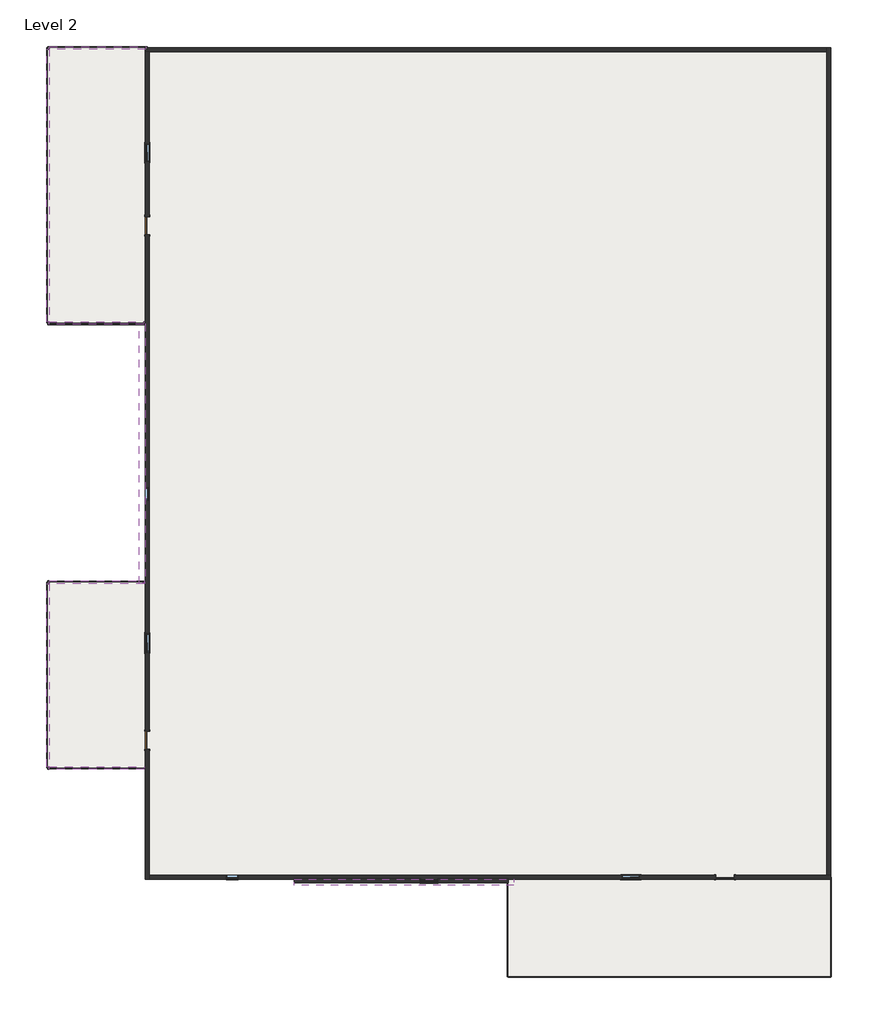
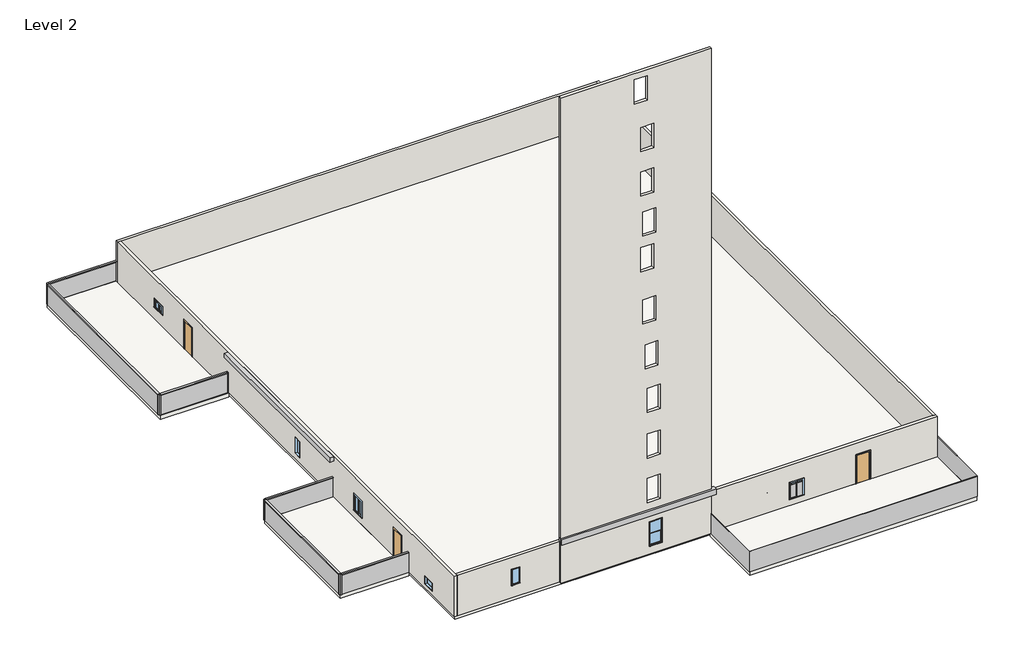
# One storey: 16 members, 10 plates, 7 windows, 5 walls, 4 slabs, 3 doors, 2 proxies.
"""IFC4 building model written with IfcOpenShell, lengths in millimetres."""

from ifc_helpers import new_model, si_unit, frame, origin, place, context, project, spatial, polyline, outline, extrude, faceted_brep, transform, mapped, element, save
from components import generic_models_11_generic_models_11_cbfe9a59, generic_models_22_generic_models_22_0e0807fa, door_54dd4da4, door_719f80de, member_4491d118, member_5d32774f, member_6474a55f, member_23f0e500, member_8787ee90, member_8a2e7db5, system_panel_glazed_dbf8c7ac, system_panel_glazed_64af9de3, system_panel_glazed_abcfc967, system_panel_glazed_a32a2426, system_panel_glazed_9b7d9a9b, system_panel_glazed_6b509a71, system_panel_glazed_fce9463a, system_panel_glazed_0e25fa2a, window_f274a882, window_80bd9af0, window_57c3ee1c, window_78885257, window_a4355bb3, window_54100e87

model = new_model("IFC4")

# Units and contexts
model_context = context("Model", 3, world=origin())
ifc_project = project(units=[si_unit("LENGTHUNIT", "METRE", prefix="MILLI")], contexts=[model_context])

# Site, building, storey
site = spatial("IfcSite", under=ifc_project)
building = spatial("IfcBuilding", under=site)
storey = spatial("IfcBuildingStorey", under=building, Name="Level 2", Elevation=3048.0)

# Proxies
placement = place(None, origin())
generic_models_11_generic_models_11_shape = generic_models_11_generic_models_11_cbfe9a59(model_context)
element("IfcBuildingElementProxy", 1, Name="Generic Models 11 : Generic Models 11", ObjectType="Generic Models 11 : Generic Models 11", at=placement, inside=storey, context=model_context, shape_type="MappedRepresentation", body=[
    mapped(generic_models_11_generic_models_11_shape, transform((0.0, 0.0, 0.0), x_axis=(1.0, 0.0, 0.0), y_axis=(0.0, 1.0, 0.0), z_axis=(0.0, 0.0, 1.0))),
])
generic_models_22_generic_models_22_shape = generic_models_22_generic_models_22_0e0807fa(model_context)
element("IfcBuildingElementProxy", 2, Name="Generic Models 22 : Generic Models 22", ObjectType="Generic Models 22 : Generic Models 22", at=placement, inside=storey, context=model_context, shape_type="MappedRepresentation", body=[
    mapped(generic_models_22_generic_models_22_shape, transform((0.0, 0.0, 0.0), x_axis=(1.0, 0.0, 0.0), y_axis=(0.0, 1.0, 0.0), z_axis=(0.0, 0.0, 1.0))),
])

# Doors
door_shape = door_54dd4da4(model_context)
element("IfcDoor", 3, ObjectType="Single-Flush : 36\" x 84\"", at=placement, inside=storey, context=model_context, shape_type="MappedRepresentation", body=[
    mapped(door_shape, transform((-15073.438074, -13886.1985361, 3048.0), x_axis=(0.0, 1.0, 0.0), y_axis=(-1.0, 0.0, 0.0), z_axis=(0.0, 0.0, 1.0))),
])
door_2_shape = door_719f80de(model_context)
element("IfcDoor", 4, ObjectType="Single-Flush : 36\" x 84\"", at=placement, inside=storey, context=model_context, shape_type="MappedRepresentation", body=[
    mapped(door_2_shape, transform((-15073.438074, 11900.6871782, 3048.0), x_axis=(0.0, -1.0, 0.0), y_axis=(1.0, 0.0, 0.0), z_axis=(0.0, 0.0, 1.0))),
])
element("IfcDoor", 5, ObjectType="Single-Flush : 36\" x 84\"", at=placement, inside=storey, context=model_context, shape_type="MappedRepresentation", body=[
    mapped(door_2_shape, transform((13882.561926, -20744.1985361, 3048.0), x_axis=(1.0, 0.0, 0.0), y_axis=(0.0, 1.0, 0.0), z_axis=(0.0, 0.0, 1.0))),
])

# Members
member_shape = member_4491d118(model_context)
element("IfcMember", 6, ObjectType="Rectangular Mullion : 2.5\" x 5\" rectangular", at=placement, inside=storey, context=model_context, shape_type="MappedRepresentation", body=[
    mapped(member_shape, transform((-20051.838074, 20810.2014639, 3048.0), x_axis=(0.0, 1.0, 0.0), y_axis=(1.0, 0.0, 0.0), z_axis=(0.0, 0.0, -1.0))),
])
element("IfcMember", 7, ObjectType="Rectangular Mullion : 2.5\" x 5\" rectangular", at=placement, inside=storey, context=model_context, shape_type="MappedRepresentation", body=[
    mapped(member_shape, transform((-15073.438074, 20810.2014639, 3048.0), x_axis=(1.0, 0.0, 0.0), y_axis=(0.0, -1.0, 0.0), z_axis=(0.0, 0.0, -1.0))),
])
element("IfcMember", 8, ObjectType="Rectangular Mullion : 2.5\" x 5\" rectangular", at=placement, inside=storey, context=model_context, shape_type="MappedRepresentation", body=[
    mapped(member_shape, transform((-20051.838074, 7023.8871782, 3048.0), x_axis=(-1.0, 0.0, 0.0), y_axis=(0.0, 1.0, 0.0), z_axis=(0.0, 0.0, -1.0))),
])
element("IfcMember", 9, ObjectType="Rectangular Mullion : 2.5\" x 5\" rectangular", at=placement, inside=storey, context=model_context, shape_type="MappedRepresentation", body=[
    mapped(member_shape, transform((-20051.838074, -5966.8213044, 3048.0), x_axis=(0.0, 1.0, 0.0), y_axis=(1.0, 0.0, 0.0), z_axis=(0.0, 0.0, -1.0))),
])
element("IfcMember", 10, ObjectType="Rectangular Mullion : 2.5\" x 5\" rectangular", at=placement, inside=storey, context=model_context, shape_type="MappedRepresentation", body=[
    mapped(member_shape, transform((-20051.838074, -15263.2213044, 3048.0), x_axis=(-1.0, 0.0, 0.0), y_axis=(0.0, 1.0, 0.0), z_axis=(0.0, 0.0, -1.0))),
])
element("IfcMember", 11, ObjectType="Rectangular Mullion : 2.5\" x 5\" rectangular", at=placement, inside=storey, context=model_context, shape_type="MappedRepresentation", body=[
    mapped(member_shape, transform((-20051.838074, 20810.2014639, 4572.0), x_axis=(-1.0, 0.0, 0.0), y_axis=(0.0, -1.0, 0.0), z_axis=(0.0, 0.0, 1.0))),
])
element("IfcMember", 12, ObjectType="Rectangular Mullion : 2.5\" x 5\" rectangular", at=placement, inside=storey, context=model_context, shape_type="MappedRepresentation", body=[
    mapped(member_shape, transform((-20051.838074, 7023.8871782, 4572.0), x_axis=(0.0, -1.0, 0.0), y_axis=(1.0, 0.0, 0.0), z_axis=(0.0, 0.0, 1.0))),
])
element("IfcMember", 13, ObjectType="Rectangular Mullion : 2.5\" x 5\" rectangular", at=placement, inside=storey, context=model_context, shape_type="MappedRepresentation", body=[
    mapped(member_shape, transform((-20051.838074, -5966.8213044, 4572.0), x_axis=(-1.0, 0.0, 0.0), y_axis=(0.0, -1.0, 0.0), z_axis=(0.0, 0.0, 1.0))),
])
element("IfcMember", 14, ObjectType="Rectangular Mullion : 2.5\" x 5\" rectangular", at=placement, inside=storey, context=model_context, shape_type="MappedRepresentation", body=[
    mapped(member_shape, transform((-20051.838074, -15263.2213044, 4572.0), x_axis=(0.0, -1.0, 0.0), y_axis=(1.0, 0.0, 0.0), z_axis=(0.0, 0.0, 1.0))),
])
element("IfcMember", 15, ObjectType="Rectangular Mullion : 2.5\" x 5\" rectangular", at=placement, inside=storey, context=model_context, shape_type="MappedRepresentation", body=[
    mapped(member_shape, transform((-15175.038074, 7023.8871782, 4572.0), x_axis=(1.0, 0.0, 0.0), y_axis=(0.0, 1.0, 0.0), z_axis=(0.0, 0.0, 1.0))),
])
member_2_shape = member_5d32774f(model_context)
element("IfcMember", 16, ObjectType="Rectangular Mullion : 2.5\" x 5\" rectangular", at=placement, inside=storey, context=model_context, shape_type="MappedRepresentation", body=[
    mapped(member_2_shape, transform((-15136.938074, 20810.2014639, 4572.0), x_axis=(0.0, 0.0, 1.0), y_axis=(0.0, -1.0, 0.0), z_axis=(1.0, 0.0, 0.0))),
])
member_3_shape = member_6474a55f(model_context)
element("IfcMember", 17, ObjectType="Rectangular Mullion : 2.5\" x 5\" rectangular", at=placement, inside=storey, context=model_context, shape_type="MappedRepresentation", body=[
    mapped(member_3_shape, transform((-20051.838074, 20746.7014639, 4572.0), x_axis=(0.0, 0.0, 1.0), y_axis=(1.0, 0.0, 0.0), z_axis=(0.0, 1.0, 0.0))),
])
member_4_shape = member_23f0e500(model_context)
element("IfcMember", 18, ObjectType="Rectangular Mullion : 2.5\" x 5\" rectangular", at=placement, inside=storey, context=model_context, shape_type="MappedRepresentation", body=[
    mapped(member_4_shape, transform((-15230.4716465, -5966.8213044, 4572.0), x_axis=(0.0, 0.0, 1.0), y_axis=(0.0, -1.0, 0.0), z_axis=(1.0, 0.0, 0.0))),
])
member_5_shape = member_8787ee90(model_context)
element("IfcMember", 19, ObjectType="Rectangular Mullion : 2.5\" x 5\" rectangular", at=placement, inside=storey, context=model_context, shape_type="MappedRepresentation", body=[
    mapped(member_5_shape, transform((-20051.838074, -6030.3213044, 4572.0), x_axis=(0.0, 0.0, 1.0), y_axis=(1.0, 0.0, 0.0), z_axis=(0.0, 1.0, 0.0))),
])
element("IfcMember", 20, ObjectType="Rectangular Mullion : 2.5\" x 5\" rectangular", at=placement, inside=storey, context=model_context, shape_type="MappedRepresentation", body=[
    mapped(member_4_shape, transform((-19988.338074, -15263.2213044, 4572.0), x_axis=(0.0, 0.0, 1.0), y_axis=(0.0, 1.0, 0.0), z_axis=(-1.0, 0.0, 0.0))),
])
member_6_shape = member_8a2e7db5(model_context)
element("IfcMember", 21, ObjectType="Rectangular Mullion : 2.5\" x 5\" rectangular", at=placement, inside=storey, context=model_context, shape_type="MappedRepresentation", body=[
    mapped(member_6_shape, transform((-19988.338074, 7023.8871782, 4572.0), x_axis=(0.0, 0.0, 1.0), y_axis=(0.0, 1.0, 0.0), z_axis=(-1.0, 0.0, 0.0))),
])

# Plates
system_panel_glazed_shape = system_panel_glazed_dbf8c7ac(model_context)
element("IfcPlate", 22, ObjectType="System Panel : Glazed", at=placement, inside=storey, context=model_context, shape_type="MappedRepresentation", body=[
    mapped(system_panel_glazed_shape, transform((11088.561926, -20845.7985361, 3048.0), x_axis=(1.0, 0.0, 0.0), y_axis=(0.0, 1.0, 0.0), z_axis=(0.0, 0.0, 1.0))),
])
element("IfcPlate", 23, ObjectType="System Panel : Glazed", at=placement, inside=storey, context=model_context, shape_type="MappedRepresentation", body=[
    mapped(system_panel_glazed_shape, transform((11088.561926, -25722.5985361, 3048.0), x_axis=(-1.0, 0.0, 0.0), y_axis=(0.0, -1.0, 0.0), z_axis=(0.0, 0.0, 1.0))),
])
system_panel_glazed_2_shape = system_panel_glazed_64af9de3(model_context)
element("IfcPlate", 24, ObjectType="System Panel : Glazed", at=placement, inside=storey, context=model_context, shape_type="MappedRepresentation", body=[
    mapped(system_panel_glazed_2_shape, transform((19165.761926, -23233.3985361, 3048.0), x_axis=(0.0, -1.0, 0.0), y_axis=(1.0, 0.0, 0.0), z_axis=(0.0, 0.0, 1.0))),
])
system_panel_glazed_3_shape = system_panel_glazed_abcfc967(model_context)
element("IfcPlate", 25, ObjectType="System Panel : Glazed", at=placement, inside=storey, context=model_context, shape_type="MappedRepresentation", body=[
    mapped(system_panel_glazed_3_shape, transform((3011.361926, -23273.4060583, 3048.0), x_axis=(0.0, 1.0, 0.0), y_axis=(-1.0, 0.0, 0.0), z_axis=(0.0, 0.0, 1.0))),
])
system_panel_glazed_4_shape = system_panel_glazed_a32a2426(model_context)
element("IfcPlate", 26, ObjectType="System Panel : Glazed", at=placement, inside=storey, context=model_context, shape_type="MappedRepresentation", body=[
    mapped(system_panel_glazed_4_shape, transform((-17562.638074, 20810.2014639, 3048.0), x_axis=(1.0, 0.0, 0.0), y_axis=(0.0, 1.0, 0.0), z_axis=(0.0, 0.0, 1.0))),
])
system_panel_glazed_5_shape = system_panel_glazed_9b7d9a9b(model_context)
element("IfcPlate", 27, ObjectType="System Panel : Glazed", at=placement, inside=storey, context=model_context, shape_type="MappedRepresentation", body=[
    mapped(system_panel_glazed_5_shape, transform((-20051.838074, 13917.0443211, 3048.0), x_axis=(0.0, 1.0, 0.0), y_axis=(-1.0, 0.0, 0.0), z_axis=(0.0, 0.0, 1.0))),
])
system_panel_glazed_6_shape = system_panel_glazed_6b509a71(model_context)
element("IfcPlate", 28, ObjectType="System Panel : Glazed", at=placement, inside=storey, context=model_context, shape_type="MappedRepresentation", body=[
    mapped(system_panel_glazed_6_shape, transform((-17609.4048602, -5966.8213044, 3048.0), x_axis=(1.0, 0.0, 0.0), y_axis=(0.0, 1.0, 0.0), z_axis=(0.0, 0.0, 1.0))),
])
element("IfcPlate", 29, ObjectType="System Panel : Glazed", at=placement, inside=storey, context=model_context, shape_type="MappedRepresentation", body=[
    mapped(system_panel_glazed_6_shape, transform((-17609.4048602, -15263.2213044, 3048.0), x_axis=(-1.0, 0.0, 0.0), y_axis=(0.0, -1.0, 0.0), z_axis=(0.0, 0.0, 1.0))),
])
system_panel_glazed_7_shape = system_panel_glazed_fce9463a(model_context)
element("IfcPlate", 30, ObjectType="System Panel : Glazed", at=placement, inside=storey, context=model_context, shape_type="MappedRepresentation", body=[
    mapped(system_panel_glazed_7_shape, transform((-20051.838074, -10615.0213044, 3048.0), x_axis=(0.0, 1.0, 0.0), y_axis=(-1.0, 0.0, 0.0), z_axis=(0.0, 0.0, 1.0))),
])
system_panel_glazed_8_shape = system_panel_glazed_0e25fa2a(model_context)
element("IfcPlate", 31, ObjectType="System Panel : Glazed", at=placement, inside=storey, context=model_context, shape_type="MappedRepresentation", body=[
    mapped(system_panel_glazed_8_shape, transform((-17613.438074, 7023.8871782, 3048.0), x_axis=(-1.0, 0.0, 0.0), y_axis=(0.0, -1.0, 0.0), z_axis=(0.0, 0.0, 1.0))),
])

# Slabs
element("IfcSlab", 32, ObjectType="Generic - 12\"", at=placement, inside=storey, context=model_context, shape_type="SweptSolid", body=[
    extrude(outline(polyline([(19064.161926, 20708.6014639), (19064.161926, -20744.1985361), (-15073.438074, -20744.1985361), (-15073.438074, 20708.6014639), (19064.161926, 20708.6014639)])), frame((0.0, 0.0, 2743.2), z_axis=(0.0, 0.0, 1.0), x_axis=(1.0, 0.0, 0.0)), (0.0, 0.0, 1.0), 304.8),
])
element("IfcSlab", 33, ObjectType="Generic - 12\"", at=placement, inside=storey, context=model_context, shape_type="SweptSolid", body=[
    extrude(outline(polyline([(3011.361926, -20845.7985361), (19165.761926, -20845.7985361), (19165.761926, -25722.5985361), (3011.361926, -25722.5985361), (3011.361926, -20845.7985361)])), frame((0.0, 0.0, 2743.2), z_axis=(0.0, 0.0, 1.0), x_axis=(1.0, 0.0, 0.0)), (0.0, 0.0, 1.0), 304.8),
])
element("IfcSlab", 34, ObjectType="Generic - 12\"", at=placement, inside=storey, context=model_context, shape_type="SweptSolid", body=[
    extrude(outline(polyline([(-20051.838074, -15263.2213044), (-20051.838074, -5966.8213044), (-15175.038074, -5966.8213044), (-15175.038074, -15263.2213044), (-20051.838074, -15263.2213044)])), frame((0.0, 0.0, 2743.2), z_axis=(0.0, 0.0, 1.0), x_axis=(1.0, 0.0, 0.0)), (0.0, 0.0, 1.0), 304.8),
])
element("IfcSlab", 35, ObjectType="Generic - 12\"", at=placement, inside=storey, context=model_context, shape_type="SweptSolid", body=[
    extrude(outline(polyline([(-20051.838074, 20810.2014639), (-15175.038074, 20810.2014639), (-15175.038074, 6941.8014639), (-20051.838074, 6941.8014639), (-20051.838074, 20810.2014639)])), frame((0.0, 0.0, 2743.2), z_axis=(0.0, 0.0, 1.0), x_axis=(1.0, 0.0, 0.0)), (0.0, 0.0, 1.0), 304.8),
])

# Walls
element("IfcWall", 36, ObjectType="Generic - 8\"", at=placement, inside=storey, context=model_context, shape_type="Brep", body=[
    faceted_brep([(-15175.038074, 20607.0014639, 3048.0), (-14971.838074, 20607.0014639, 3048.0), (18962.561926, 20607.0014639, 3048.0), (18962.561926, 20607.0014639, 6096.0), (-14971.838074, 20607.0014639, 6096.0), (-15175.038074, 20607.0014639, 6096.0), (-15175.038074, 20810.2014639, 3048.0), (-15175.038074, 20810.2014639, 6096.0), (18962.561926, 20810.2014639, 6096.0), (18962.561926, 20810.2014639, 3048.0)], [[[0, 1, 2, 3, 4, 5]], [[6, 7, 8, 9]], [[2, 1, 0, 6, 9]], [[5, 4, 3, 8, 7]], [[0, 5, 7, 6]], [[3, 2, 9, 8]]]),
])
element("IfcWall", 37, ObjectType="Generic - 8\"", at=placement, inside=storey, context=model_context, shape_type="Brep", body=[
    faceted_brep([(-14971.838074, -13428.9985361, 5181.6), (-14971.838074, -13428.9985361, 3048.0), (-14971.838074, 11443.4871782, 3048.0), (-14971.838074, 11443.4871782, 5181.6), (-14971.838074, 12357.8871782, 5181.6), (-14971.838074, 12357.8871782, 3048.0), (-14971.838074, 20607.0014639, 3048.0), (-14971.838074, 20607.0014639, 6096.0), (-14971.838074, -20642.5985361, 6096.0), (-14971.838074, -20845.7985361, 6096.0), (-14971.838074, -20845.7985361, 3048.0), (-14971.838074, -20642.5985361, 3048.0), (-14971.838074, -14343.3985361, 3048.0), (-14971.838074, -14343.3985361, 5181.6), (-14971.838074, -8552.1985361, 4802.6417877), (-14971.838074, -8552.1985361, 3583.4417877), (-14971.838074, -9466.5985361, 3583.4417877), (-14971.838074, -9466.5985361, 4802.6417877), (-14971.838074, -1846.5985361, 4692.1881061), (-14971.838074, -1236.9985361, 4692.1881061), (-14971.838074, -1236.9985361, 3472.9881061), (-14971.838074, -1846.5985361, 3472.9881061), (-14971.838074, 16015.4871782, 4572.0), (-14971.838074, 16015.4871782, 3962.4), (-14971.838074, 15101.0871782, 3962.4), (-14971.838074, 15101.0871782, 4572.0), (-14971.838074, -18153.3985361, 3943.5283704), (-14971.838074, -17238.9985361, 3943.5283704), (-14971.838074, -17238.9985361, 3333.9283704), (-14971.838074, -18153.3985361, 3333.9283704), (-15175.038074, 11443.4871782, 3048.0), (-15175.038074, -13428.9985361, 3048.0), (-15175.038074, -13428.9985361, 5181.6), (-15175.038074, -14343.3985361, 5181.6), (-15175.038074, -14343.3985361, 3048.0), (-15175.038074, -20845.7985361, 3048.0), (-15175.038074, -20845.7985361, 6096.0), (-15175.038074, 20607.0014639, 6096.0), (-15175.038074, 20607.0014639, 3048.0), (-15175.038074, 12357.8871782, 3048.0), (-15175.038074, 12357.8871782, 5181.6), (-15175.038074, 11443.4871782, 5181.6), (-15175.038074, -8552.1985361, 4802.6417877), (-15175.038074, -9466.5985361, 4802.6417877), (-15175.038074, -9466.5985361, 3583.4417877), (-15175.038074, -8552.1985361, 3583.4417877), (-15175.038074, -1846.5985361, 4692.1881061), (-15175.038074, -1846.5985361, 3472.9881061), (-15175.038074, -1236.9985361, 3472.9881061), (-15175.038074, -1236.9985361, 4692.1881061), (-15175.038074, 16015.4871782, 4572.0), (-15175.038074, 15101.0871782, 4572.0), (-15175.038074, 15101.0871782, 3962.4), (-15175.038074, 16015.4871782, 3962.4), (-15175.038074, -18153.3985361, 3943.5283704), (-15175.038074, -18153.3985361, 3333.9283704), (-15175.038074, -17238.9985361, 3333.9283704), (-15175.038074, -17238.9985361, 3943.5283704)], [[[0, 1, 2, 3, 4, 5, 6, 7, 8, 9, 10, 11, 12, 13], [14, 15, 16, 17], [18, 19, 20, 21], [22, 23, 24, 25], [26, 27, 28, 29]], [[30, 31, 32, 33, 34, 35, 36, 37, 38, 39, 40, 41], [42, 43, 44, 45], [46, 47, 48, 49], [50, 51, 52, 53], [54, 55, 56, 57]], [[39, 38, 6, 5]], [[2, 1, 31, 30]], [[12, 11, 10, 35, 34]], [[9, 8, 7, 37, 36]], [[10, 9, 36, 35]], [[7, 6, 38, 37]], [[3, 2, 30, 41]], [[4, 3, 41, 40]], [[5, 4, 40, 39]], [[32, 31, 1, 0]], [[33, 32, 0, 13]], [[34, 33, 13, 12]], [[15, 14, 42, 45]], [[16, 15, 45, 44]], [[17, 16, 44, 43]], [[14, 17, 43, 42]], [[47, 46, 18, 21]], [[48, 47, 21, 20]], [[49, 48, 20, 19]], [[46, 49, 19, 18]], [[23, 22, 50, 53]], [[24, 23, 53, 52]], [[25, 24, 52, 51]], [[22, 25, 51, 50]], [[55, 54, 26, 29]], [[56, 55, 29, 28]], [[57, 56, 28, 27]], [[54, 57, 27, 26]]]),
])
element("IfcWall", 38, ObjectType="Generic - 8\"", at=placement, inside=storey, context=model_context, shape_type="Brep", body=[
    faceted_brep([(19165.761926, -20642.5985361, 3048.0), (18962.561926, -20642.5985361, 3048.0), (14339.761926, -20642.5985361, 3048.0), (14339.761926, -20642.5985361, 5181.6), (13425.361926, -20642.5985361, 5181.6), (13425.361926, -20642.5985361, 3048.0), (-14971.838074, -20642.5985361, 3048.0), (-14971.838074, -20642.5985361, 6096.0), (18962.561926, -20642.5985361, 6096.0), (19165.761926, -20642.5985361, 6096.0), (-11111.038074, -20642.5985361, 5181.6), (-11111.038074, -20642.5985361, 3962.4), (-10501.438074, -20642.5985361, 3962.4), (-10501.438074, -20642.5985361, 5181.6), (8700.961926, -20642.5985361, 4744.0997669), (8700.961926, -20642.5985361, 3524.8997669), (9615.361926, -20642.5985361, 3524.8997669), (9615.361926, -20642.5985361, 4744.0997669), (14339.761926, -20845.7985361, 5181.6), (14339.761926, -20845.7985361, 3048.0), (19165.761926, -20845.7985361, 3048.0), (19165.761926, -20845.7985361, 6096.0), (-14971.838074, -20845.7985361, 6096.0), (-14971.838074, -20845.7985361, 3048.0), (13425.361926, -20845.7985361, 3048.0), (13425.361926, -20845.7985361, 5181.6), (-11111.038074, -20845.7985361, 5181.6), (-10501.438074, -20845.7985361, 5181.6), (-10501.438074, -20845.7985361, 3962.4), (-11111.038074, -20845.7985361, 3962.4), (8700.961926, -20845.7985361, 4744.0997669), (9615.361926, -20845.7985361, 4744.0997669), (9615.361926, -20845.7985361, 3524.8997669), (8700.961926, -20845.7985361, 3524.8997669)], [[[0, 1, 2, 3, 4, 5, 6, 7, 8, 9], [10, 11, 12, 13], [14, 15, 16, 17]], [[18, 19, 20, 21, 22, 23, 24, 25], [26, 27, 28, 29], [30, 31, 32, 33]], [[24, 23, 6, 5]], [[20, 19, 2, 1, 0]], [[9, 8, 7, 22, 21]], [[0, 9, 21, 20]], [[7, 6, 23, 22]], [[3, 2, 19, 18]], [[4, 3, 18, 25]], [[5, 4, 25, 24]], [[11, 10, 26, 29]], [[12, 11, 29, 28]], [[13, 12, 28, 27]], [[10, 13, 27, 26]], [[15, 14, 30, 33]], [[16, 15, 33, 32]], [[17, 16, 32, 31]], [[14, 17, 31, 30]]]),
])
element("IfcWall", 39, ObjectType="Generic - 8\"", at=placement, inside=storey, context=model_context, shape_type="Brep", body=[
    faceted_brep([(18962.561926, 20810.2014639, 3048.0), (18962.561926, 20607.0014639, 3048.0), (18962.561926, -20642.5985361, 3048.0), (18962.561926, -20642.5985361, 6096.0), (18962.561926, 20607.0014639, 6096.0), (18962.561926, 20810.2014639, 6096.0), (19165.761926, 20810.2014639, 3048.0), (19165.761926, 20810.2014639, 6096.0), (19165.761926, -20642.5985361, 6096.0), (19165.761926, -20642.5985361, 3048.0)], [[[0, 1, 2, 3, 4, 5]], [[6, 7, 8, 9]], [[2, 1, 0, 6, 9]], [[5, 4, 3, 8, 7]], [[0, 5, 7, 6]], [[3, 2, 9, 8]]]),
])
element("IfcWall", 40, ObjectType="Generic - 8\"", at=placement, inside=storey, context=model_context, shape_type="SweptSolid", body=[
    extrude(outline(polyline([(3048.0, 3011.361926), (39560.282979, 3011.361926), (39560.282979, -7701.088074), (3048.0, -7701.088074), (3048.0, 3011.361926)]), holes=[polyline([(39093.913115, -2475.038074), (39093.913115, -1560.638074), (37265.113115, -1560.638074), (37265.113115, -2475.038074), (39093.913115, -2475.038074)]), polyline([(35356.8, -2017.838074), (35356.8, -1103.438074), (33528.0, -1103.438074), (33528.0, -2017.838074), (35356.8, -2017.838074)]), polyline([(32004.0, -2017.838074), (32004.0, -1103.438074), (30175.2, -1103.438074), (30175.2, -2017.838074), (32004.0, -2017.838074)]), polyline([(26301.0535848, -2017.838074), (26301.0535848, -1103.438074), (24472.2535848, -1103.438074), (24472.2535848, -2017.838074), (26301.0535848, -2017.838074)]), polyline([(28940.5086033, -1865.438074), (28940.5086033, -951.038074), (27111.7086033, -951.038074), (27111.7086033, -1865.438074), (28940.5086033, -1865.438074)]), polyline([(22326.1798521, -1865.438074), (22326.1798521, -951.038074), (20497.3798521, -951.038074), (20497.3798521, -1865.438074), (22326.1798521, -1865.438074)]), polyline([(18897.3012618, -1713.038074), (18897.3012618, -798.638074), (17068.5012618, -798.638074), (17068.5012618, -1713.038074), (18897.3012618, -1713.038074)]), polyline([(15577.0516227, -1560.638074), (15577.0516227, -646.238074), (13748.2516227, -646.238074), (13748.2516227, -1560.638074), (15577.0516227, -1560.638074)]), polyline([(12131.0772003, -1560.638074), (12131.0772003, -646.238074), (10302.2772003, -646.238074), (10302.2772003, -1560.638074), (12131.0772003, -1560.638074)]), polyline([(8798.7958658, -1560.638074), (8798.7958658, -646.238074), (6969.9958658, -646.238074), (6969.9958658, -1560.638074), (8798.7958658, -1560.638074)]), polyline([(5470.6482063, -1408.238074), (5470.6482063, -493.838074), (3641.8482063, -493.838074), (3641.8482063, -1408.238074), (5470.6482063, -1408.238074)])]), frame((0.0, -21023.5985361, 0.0), z_axis=(0.0, 1.0, 0.0), x_axis=(0.0, 0.0, 1.0)), (0.0, 0.0, 1.0), 203.2),
])

# Windows
window_shape = window_f274a882(model_context)
element("IfcWindow", 41, ObjectType="Double Hung : 36\" x 72\"", at=placement, inside=storey, context=model_context, shape_type="MappedRepresentation", body=[
    mapped(window_shape, transform((-951.038074, -20921.9985361, 3337.0482063), x_axis=(-1.0, 0.0, 0.0), y_axis=(0.0, -1.0, 0.0), z_axis=(0.0, 0.0, 1.0))),
])
window_2_shape = window_80bd9af0(model_context)
element("IfcWindow", 42, ObjectType="Fixed : 24\" x 48\"", at=placement, inside=storey, context=model_context, shape_type="MappedRepresentation", body=[
    mapped(window_2_shape, transform((-15073.438074, -1579.8985361, 2558.5881061), x_axis=(0.0, -1.0, 0.0), y_axis=(1.0, 0.0, 0.0), z_axis=(0.0, 0.0, 1.0))),
])
window_3_shape = window_57c3ee1c(model_context)
element("IfcWindow", 43, ObjectType="Fixed : 36\" x 24\"", at=placement, inside=storey, context=model_context, shape_type="MappedRepresentation", body=[
    mapped(window_3_shape, transform((-15073.438074, -17734.2985361, 2419.5283704), x_axis=(0.0, -1.0, 0.0), y_axis=(1.0, 0.0, 0.0), z_axis=(0.0, 0.0, 1.0))),
])
window_4_shape = window_78885257(model_context)
element("IfcWindow", 44, ObjectType="Instance - Fixed : 24\" x 48\"", at=placement, inside=storey, context=model_context, shape_type="MappedRepresentation", body=[
    mapped(window_4_shape, transform((-10844.338074, -20744.1985361, 3048.0), x_axis=(-1.0, 0.0, 0.0), y_axis=(0.0, -1.0, 0.0), z_axis=(0.0, 0.0, 1.0))),
])
window_5_shape = window_a4355bb3(model_context)
element("IfcWindow", 45, ObjectType="Slider with Trim : 36\" x 24\"", at=placement, inside=storey, context=model_context, shape_type="MappedRepresentation", body=[
    mapped(window_5_shape, transform((-15073.438074, 15558.2871782, 3048.0), x_axis=(0.0, 1.0, 0.0), y_axis=(-1.0, 0.0, 0.0), z_axis=(0.0, 0.0, 1.0))),
])
window_6_shape = window_54100e87(model_context)
element("IfcWindow", 46, ObjectType="Slider with Trim : 36\" x 48\"", at=placement, inside=storey, context=model_context, shape_type="MappedRepresentation", body=[
    mapped(window_6_shape, transform((9158.161926, -20744.1985361, 2610.4997669), x_axis=(-1.0, 0.0, 0.0), y_axis=(0.0, -1.0, 0.0), z_axis=(0.0, 0.0, 1.0))),
])
element("IfcWindow", 47, ObjectType="Slider with Trim : 36\" x 48\"", at=placement, inside=storey, context=model_context, shape_type="MappedRepresentation", body=[
    mapped(window_6_shape, transform((-15073.438074, -9009.3985361, 2669.0417877), x_axis=(0.0, 1.0, 0.0), y_axis=(-1.0, 0.0, 0.0), z_axis=(0.0, 0.0, 1.0))),
])

save(model, "model.ifc")

# Revit data of these elements
# Type "Single-Flush : 36\" x 84\""
#   Type Mark = "1"
#   Construction Type Id = "MDOOR"
#   Assembly Code = "C1020"
#   Analytic Construction = "Metal"
#   Thickness = 0' - 2"
#   Heat Transfer Coefficient (U) = 0.651978 BTU/(h·ft²·°F)
#   Height = 7' - 0"
#   Trim Projection Ext = 0' - 1"
#   Trim Projection Int = 0' - 1"
#   Trim Width = 0' - 3"
#   Width = 3' - 0"
#   Define Thermal Properties by = 1
#   Door Material = Door - Panel
#   Frame Material = Door - Frame
#   Visual Light Transmittance = 0
#   Solar Heat Gain Coefficient = 0
#   Function = (empty or 0)
#   Wall Closure = (empty or 0)
# Type "Rectangular Mullion : 2.5\" x 5\" rectangular"
#   built-in parameter 1007304 = 0.416667 (stored number, unit not read)
#   built-in parameter 1007301 = 0.104167 (stored number, unit not read)
#   built-in parameter 1007300 = 0.104167 (stored number, unit not read)
# Type "System Panel : Glazed"
#   Construction Type Id = "GSP4R"
#   Analytic Construction = "1/8 in Pilkington single glazing"
#   Visual Light Transmittance = 0.9
#   Solar Heat Gain Coefficient = 0.86
#   Heat Transfer Coefficient (U) = 1.18115 BTU/(h·ft²·°F)
# Type "Generic - 12\""
#   Assembly Code = "B1010"
#   Function = 0
#   Layers, outside or top first: 1' - 0" no material (function 1)
# Type "Generic - 8\""
#   Assembly Code = "B2010"
#   Layers, outside or top first: 0' - 8" no material (function 1)
# Type "Double Hung : 36\" x 72\""
#   Type Mark = "18"
#   Construction Type Id = "GSP4R"
#   Assembly Code = "B2020100"
#   Analytic Construction = "1/8 in Pilkington single glazing"
#   Visual Light Transmittance = 0.9
#   Solar Heat Gain Coefficient = 0.78
#   Heat Transfer Coefficient (U) = 0.6496 BTU/(h·ft²·°F)
#   Height = 6' - 0"
#   Default Sill Height = 1' - 0"
#   Width = 3' - 0"
#   Window Inset = 0' - 0 3/4"
#   Define Thermal Properties by = 1
#   Glass Pane Material = Glass
#   Sash Material = Sash
#   Description = (empty or 0)
#   Wall Closure = (empty or 0)
# Type "Fixed : 24\" x 48\""
#   Type Mark = "2"
#   Construction Type Id = "GSP4R"
#   Assembly Code = "B2020100"
#   Analytic Construction = "1/8 in Pilkington single glazing"
#   Visual Light Transmittance = 0.9
#   Solar Heat Gain Coefficient = 0.78
#   Heat Transfer Coefficient (U) = 0.6496 BTU/(h·ft²·°F)
#   Height = 4' - 0"
#   Default Sill Height = 3' - 0"
#   Width = 2' - 0"
#   Window Inset = 0' - 0 3/4"
#   Define Thermal Properties by = 1
#   Glass Pane Material = Glass
#   Sash Material = Sash
#   Wall Closure = (empty or 0)
# Type "Fixed : 36\" x 24\""
#   Type Mark = "8"
#   Construction Type Id = "GSP4R"
#   Assembly Code = "B2020100"
#   Analytic Construction = "1/8 in Pilkington single glazing"
#   Visual Light Transmittance = 0.9
#   Solar Heat Gain Coefficient = 0.78
#   Heat Transfer Coefficient (U) = 0.6496 BTU/(h·ft²·°F)
#   Height = 2' - 0"
#   Default Sill Height = 3' - 0"
#   Width = 3' - 0"
#   Window Inset = 0' - 0 3/4"
#   Define Thermal Properties by = 1
#   Glass Pane Material = Glass
#   Sash Material = Sash
#   Wall Closure = (empty or 0)
# Type "Instance - Fixed : 24\" x 48\""
#   Type Mark = "19"
#   Construction Type Id = "GSP4R"
#   Assembly Code = "B2020100"
#   Analytic Construction = "1/8 in Pilkington single glazing"
#   Visual Light Transmittance = 0.9
#   Thermal Resistance (R) = 0.8466 (h·ft²·°F)/BTU
#   Solar Heat Gain Coefficient = 0.86
#   Heat Transfer Coefficient (U) = 1.1812 BTU/(h·ft²·°F)
#   Height [instance default] = 4' - 0"
#   Default Sill Height = 3' - 0"
#   Width [instance default] = 2' - 0"
#   Window Inset = 0' - 0 3/4"
#   Define Thermal Properties by = 1
#   Glass Pane Material = Glass
#   Sash Material = Sash
#   Wall Closure = (empty or 0)
# Type "Slider with Trim : 36\" x 24\""
#   Type Mark = "23"
#   Construction Type Id = "GSP4R"
#   Assembly Code = "B2020100"
#   Analytic Construction = "1/8 in Pilkington single glazing"
#   Visual Light Transmittance = 0.9
#   Solar Heat Gain Coefficient = 0.78
#   Heat Transfer Coefficient (U) = 0.6496 BTU/(h·ft²·°F)
#   Height = 2' - 0"
#   Default Sill Height = 3' - 0"
#   Trim Projection - Ext. = 0' - 0 3/4"
#   Trim Projection - Int. = 0' - 0 3/4"
#   Trim Width - Exterior = 0' - 3 1/2"
#   Trim Width - Interior = 0' - 3 1/2"
#   Width = 3' - 0"
#   Window Inset = 0' - 0 3/4"
#   Define Thermal Properties by = 1
#   Glass Pane Material = Glass
#   Sash Material = Sash
#   Trim Exterior Material = Trim
#   Trim Interior Material = Trim
#   Wall Closure = (empty or 0)
# Type "Slider with Trim : 36\" x 48\""
#   Type Mark = "22"
#   Construction Type Id = "GSP4R"
#   Assembly Code = "B2020100"
#   Analytic Construction = "1/8 in Pilkington single glazing"
#   Visual Light Transmittance = 0.9
#   Solar Heat Gain Coefficient = 0.78
#   Heat Transfer Coefficient (U) = 0.6496 BTU/(h·ft²·°F)
#   Height = 4' - 0"
#   Default Sill Height = 3' - 0"
#   Trim Projection - Ext. = 0' - 0 3/4"
#   Trim Projection - Int. = 0' - 0 3/4"
#   Trim Width - Exterior = 0' - 3 1/2"
#   Trim Width - Interior = 0' - 3 1/2"
#   Width = 3' - 0"
#   Window Inset = 0' - 0 3/4"
#   Define Thermal Properties by = 1
#   Glass Pane Material = Glass
#   Sash Material = Sash
#   Trim Exterior Material = Trim
#   Trim Interior Material = Trim
#   Wall Closure = (empty or 0)
# Element 1 (IfcBuildingElementProxy, "Generic Models 11 : Generic Models 11")
#   Phase Created = New Construction
# Element 2 (IfcBuildingElementProxy, "Generic Models 22 : Generic Models 22")
#   Phase Created = New Construction
# Elements 3, 4, 5 (IfcDoor, "Single-Flush : 36\" x 84\"")
#   Phase Created = New Construction
#   Materials on its faces: "Door - Frame", "Door - Panel"
# Elements 6, 7, 8, 9, 10, 11, 12, 13, 14, 15, 16, 17, 18, 19, 20, 21 (IfcMember, "Rectangular Mullion : 2.5\" x 5\" rectangular")
#   Phase Created = New Construction
#   Materials on its faces: "Aluminum"
# Elements 22, 23, 24, 25, 26, 27, 28, 29, 30, 31 (IfcPlate, "System Panel : Glazed")
#   Phase Created = New Construction
#   Materials on its faces: "Glass"
# Element 32 (IfcSlab, "Generic - 12\"")
#   Height Offset From Level = 0' - 0"
#   Phase Created = New Construction
#   Materials on its faces: "Default Floor"
# Elements 33, 34, 35 (IfcSlab, "Generic - 12\"")
#   built-in parameter 1001955 = 3.14159 (stored number, unit not read)
#   Height Offset From Level = 0' - 0"
#   Phase Created = New Construction
#   Materials on its faces: "Default Floor"
# Elements 36, 37, 38, 39 (IfcWall, "Generic - 8\"")
#   Top Offset = 0' - 0"
#   Base Offset = 0' - 0"
#   Unconnected Height = 10' - 0"
#   wall height = 10' - 0"
#   Phase Created = New Construction
#   Base Constraint = Level 2
#   Materials on its faces: "Default Wall"
# Element 40 (IfcWall, "Generic - 8\"")
#   Top Offset = 0' - 0"
#   Base Offset = 0' - 0"
#   Unconnected Height = 119' - 9.49146"
#   wall height = 119' - 9.49146"
#   Phase Created = New Construction
#   Base Constraint = Level 2
#   Materials on its faces: "Default Wall"
# Element 41 (IfcWindow, "Double Hung : 36\" x 72\"")
#   Mark = "11"
#   Phase Created = New Construction
#   Materials on its faces: "Sash", "Glass"
# Element 42 (IfcWindow, "Fixed : 24\" x 48\"")
#   Mark = "55"
#   Phase Created = New Construction
#   Materials on its faces: "Sash", "Glass"
# Element 43 (IfcWindow, "Fixed : 36\" x 24\"")
#   Mark = "77"
#   Phase Created = New Construction
#   Materials on its faces: "Sash", "Glass"
# Element 44 (IfcWindow, "Instance - Fixed : 24\" x 48\"")
#   Mark = "22"
#   Width = 2' - 0"
#   Height = 4' - 0"
#   Phase Created = New Construction
#   Materials on its faces: "Sash", "Glass"
# Element 45 (IfcWindow, "Slider with Trim : 36\" x 24\"")
#   Mark = "66"
#   Phase Created = New Construction
#   Materials on its faces: "Sash", "Trim", "Glass"
# Element 46 (IfcWindow, "Slider with Trim : 36\" x 48\"")
#   Mark = "33"
#   Phase Created = New Construction
#   Materials on its faces: "Sash", "Trim", "Glass"
# Element 47 (IfcWindow, "Slider with Trim : 36\" x 48\"")
#   Mark = "44"
#   Phase Created = New Construction
#   Materials on its faces: "Sash", "Trim", "Glass"
# Materials
#   "Door - Panel": class "Wood", colour RGB 210 159 95, transparency 0
#   "Door - Frame": colour RGB 118 70 51, transparency 0
#   "Glass": class "Glass", colour RGB 0 128 192, transparency 0.75, Description = "Soda Lime Glass", Cost = 0
#   "Sash": class "Wood", colour RGB 224 178 126, transparency 0
#   "Trim": class "Wood", colour RGB 224 178 126, transparency 0
#   "Aluminum": class "Metal", colour RGB 247 247 247, transparency 0, Description = "Aluminum 6061", Cost = 0
#   "Default Floor": colour RGB 128 128 128, transparency 0
#   "Default Wall": colour RGB 128 128 128, transparency 0
